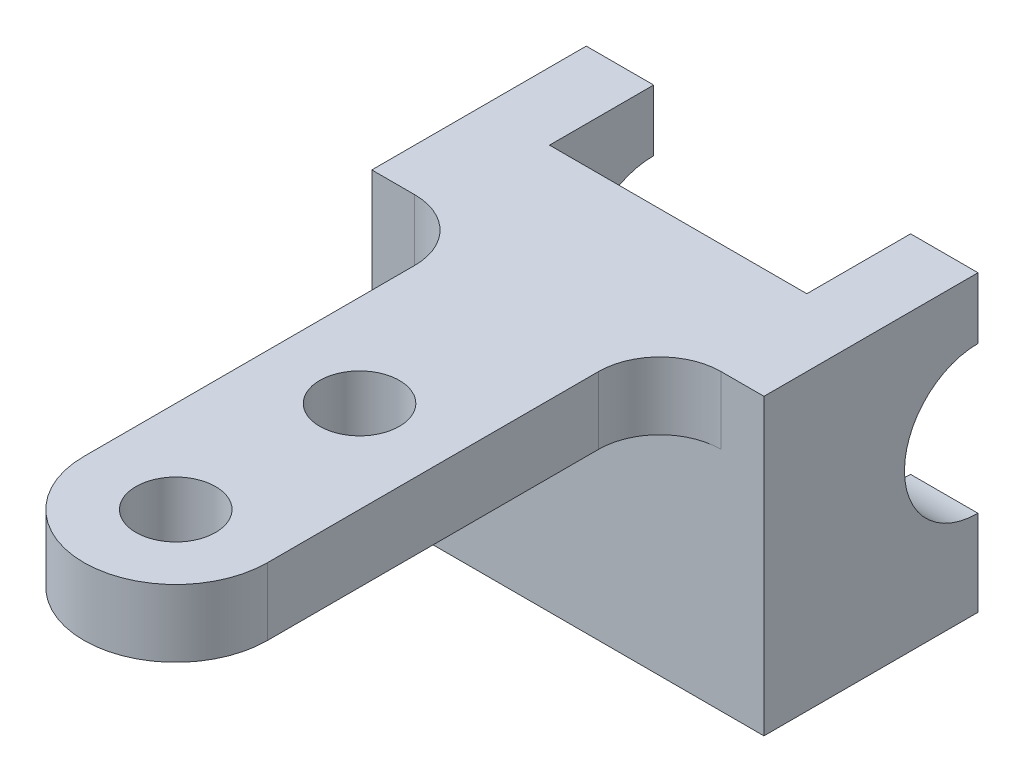
ISO-10303-21;
HEADER;
FILE_DESCRIPTION(('STEP AP214'),'2;1');
FILE_NAME('part.step','',(''),(''),'','','');
FILE_SCHEMA(('AUTOMOTIVE_DESIGN { 1 0 10303 214 1 1 1 1 }'));
ENDSEC;
DATA;
#1=APPLICATION_CONTEXT('core data for automotive mechanical design processes');
#2=APPLICATION_PROTOCOL_DEFINITION('international standard','automotive_design',2000,#1);
#3=PRODUCT_CONTEXT('',#1,'mechanical');
#4=PRODUCT('Part','Part','',(#3));
#5=PRODUCT_RELATED_PRODUCT_CATEGORY('part','',(#4));
#6=PRODUCT_DEFINITION_FORMATION('','',#4);
#7=PRODUCT_DEFINITION_CONTEXT('part definition',#1,'design');
#8=PRODUCT_DEFINITION('design','',#6,#7);
#9=PRODUCT_DEFINITION_SHAPE('','',#8);
#10=(LENGTH_UNIT() NAMED_UNIT(*) SI_UNIT(.MILLI.,.METRE.));
#11=(NAMED_UNIT(*) PLANE_ANGLE_UNIT() SI_UNIT($,.RADIAN.));
#12=(NAMED_UNIT(*) SI_UNIT($,.STERADIAN.) SOLID_ANGLE_UNIT());
#13=UNCERTAINTY_MEASURE_WITH_UNIT(LENGTH_MEASURE(1.E-05),#10,'distance_accuracy_value','');
#14=(GEOMETRIC_REPRESENTATION_CONTEXT(3) GLOBAL_UNCERTAINTY_ASSIGNED_CONTEXT((#13)) GLOBAL_UNIT_ASSIGNED_CONTEXT((#10,
#11,#12)) REPRESENTATION_CONTEXT('',''));
#15=CARTESIAN_POINT('',(0.,0.,0.));
#16=DIRECTION('',(0.,0.,1.));
#17=DIRECTION('',(1.,0.,0.));
#18=AXIS2_PLACEMENT_3D('',#15,#16,#17);
#19=CARTESIAN_POINT('',(32.,11.,-64.));
#20=DIRECTION('',(-1.,0.,0.));
#21=DIRECTION('',(0.,0.,1.));
#22=AXIS2_PLACEMENT_3D('',#19,#20,#21);
#23=PLANE('',#22);
#24=CARTESIAN_POINT('',(32.000012,-11.,-98.9340644485926));
#25=DIRECTION('',(1.,0.,0.));
#26=DIRECTION('',(0.,1.,2.23257407931203E-09));
#27=AXIS2_PLACEMENT_3D('',#24,#25,#26);
#28=CIRCLE('',#27,12.);
#29=CARTESIAN_POINT('',(32.000006,0.99999999999999,-98.9340644351971));
#30=VERTEX_POINT('',#29);
#31=CARTESIAN_POINT('',(32.000006,-23.,-98.9340644560229));
#32=VERTEX_POINT('',#31);
#33=EDGE_CURVE('E184',#30,#32,#28,.T.);
#34=ORIENTED_EDGE('',*,*,#33,.F.);
#35=DIRECTION('',(0.,-1.,0.));
#36=VECTOR('',#35,1.);
#37=CARTESIAN_POINT('',(32.,11.,-98.9340644485926));
#38=LINE('',#37,#36);
#39=CARTESIAN_POINT('',(32.,11.,-98.9340644485926));
#40=VERTEX_POINT('',#39);
#41=EDGE_CURVE('E216',#40,#30,#38,.T.);
#42=ORIENTED_EDGE('',*,*,#41,.F.);
#43=DIRECTION('',(0.,0.,-1.));
#44=VECTOR('',#43,1.);
#45=CARTESIAN_POINT('',(32.,11.,-64.));
#46=LINE('',#45,#44);
#47=CARTESIAN_POINT('',(32.,11.,-64.));
#48=VERTEX_POINT('',#47);
#49=EDGE_CURVE('E253',#48,#40,#46,.T.);
#50=ORIENTED_EDGE('',*,*,#49,.F.);
#51=DIRECTION('',(0.,-1.,0.));
#52=VECTOR('',#51,1.);
#53=CARTESIAN_POINT('',(32.,11.,-64.));
#54=LINE('',#53,#52);
#55=CARTESIAN_POINT('',(32.,-37.,-64.));
#56=VERTEX_POINT('',#55);
#57=EDGE_CURVE('E211',#48,#56,#54,.T.);
#58=ORIENTED_EDGE('',*,*,#57,.T.);
#59=DIRECTION('',(0.,0.,1.));
#60=VECTOR('',#59,1.);
#61=CARTESIAN_POINT('',(32.,-37.,-64.));
#62=LINE('',#61,#60);
#63=CARTESIAN_POINT('',(32.,-37.,-98.9340644485926));
#64=VERTEX_POINT('',#63);
#65=EDGE_CURVE('E246',#64,#56,#62,.T.);
#66=ORIENTED_EDGE('',*,*,#65,.F.);
#67=EDGE_CURVE('E208',#32,#64,#38,.T.);
#68=ORIENTED_EDGE('',*,*,#67,.F.);
#69=EDGE_LOOP('',(#34,#42,#50,#58,#66,#68));
#70=FACE_BOUND('',#69,.T.);
#71=ADVANCED_FACE('F39',(#70),#23,.F.);
#72=CARTESIAN_POINT('',(32.,11.,-98.9340644485926));
#73=DIRECTION('',(0.,0.,1.));
#74=DIRECTION('',(1.,0.,0.));
#75=AXIS2_PLACEMENT_3D('',#72,#73,#74);
#76=PLANE('',#75);
#77=DIRECTION('',(0.,-1.,0.));
#78=VECTOR('',#77,1.);
#79=CARTESIAN_POINT('',(21.,11.,-98.9340644485926));
#80=LINE('',#79,#78);
#81=CARTESIAN_POINT('',(21.,-23.,-98.9340644485926));
#82=VERTEX_POINT('',#81);
#83=CARTESIAN_POINT('',(21.,-37.,-98.9340644485926));
#84=VERTEX_POINT('',#83);
#85=EDGE_CURVE('E204',#82,#84,#80,.T.);
#86=ORIENTED_EDGE('',*,*,#85,.F.);
#87=DIRECTION('',(1.,0.,0.));
#88=VECTOR('',#87,1.);
#89=CARTESIAN_POINT('',(-32.,-23.,-98.9340644485926));
#90=LINE('',#89,#88);
#91=EDGE_CURVE('E59',#82,#32,#90,.T.);
#92=ORIENTED_EDGE('',*,*,#91,.T.);
#93=ORIENTED_EDGE('',*,*,#67,.T.);
#94=DIRECTION('',(1.,0.,0.));
#95=VECTOR('',#94,1.);
#96=CARTESIAN_POINT('',(32.,-37.,-98.9340644485926));
#97=LINE('',#96,#95);
#98=EDGE_CURVE('E265',#84,#64,#97,.T.);
#99=ORIENTED_EDGE('',*,*,#98,.F.);
#100=EDGE_LOOP('',(#86,#92,#93,#99));
#101=FACE_BOUND('',#100,.T.);
#102=ADVANCED_FACE('F351',(#101),#76,.F.);
#103=CARTESIAN_POINT('',(-21.,11.,-99.));
#104=DIRECTION('',(0.,0.,1.));
#105=DIRECTION('',(1.,0.,0.));
#106=AXIS2_PLACEMENT_3D('',#103,#104,#105);
#107=PLANE('',#106);
#108=DIRECTION('',(0.,-1.,0.));
#109=VECTOR('',#108,1.);
#110=CARTESIAN_POINT('',(-32.,11.,-99.));
#111=LINE('',#110,#109);
#112=CARTESIAN_POINT('',(-32.,-22.9998188529269,-99.));
#113=VERTEX_POINT('',#112);
#114=CARTESIAN_POINT('',(-32.,-37.,-99.));
#115=VERTEX_POINT('',#114);
#116=EDGE_CURVE('E179',#113,#115,#111,.T.);
#117=ORIENTED_EDGE('',*,*,#116,.F.);
#118=DIRECTION('',(1.,0.,0.));
#119=VECTOR('',#118,1.);
#120=CARTESIAN_POINT('',(-32.,-22.9998188529269,-99.));
#121=LINE('',#120,#119);
#122=CARTESIAN_POINT('',(-21.,-22.9998188529269,-99.));
#123=VERTEX_POINT('',#122);
#124=EDGE_CURVE('E164',#113,#123,#121,.T.);
#125=ORIENTED_EDGE('',*,*,#124,.T.);
#126=DIRECTION('',(0.,-1.,0.));
#127=VECTOR('',#126,1.);
#128=CARTESIAN_POINT('',(-21.,11.,-99.));
#129=LINE('',#128,#127);
#130=CARTESIAN_POINT('',(-21.,-37.,-99.));
#131=VERTEX_POINT('',#130);
#132=EDGE_CURVE('E195',#123,#131,#129,.T.);
#133=ORIENTED_EDGE('',*,*,#132,.T.);
#134=DIRECTION('',(1.,0.,0.));
#135=VECTOR('',#134,1.);
#136=CARTESIAN_POINT('',(-21.,-37.,-99.));
#137=LINE('',#136,#135);
#138=EDGE_CURVE('E186',#115,#131,#137,.T.);
#139=ORIENTED_EDGE('',*,*,#138,.F.);
#140=EDGE_LOOP('',(#117,#125,#133,#139));
#141=FACE_BOUND('',#140,.T.);
#142=ADVANCED_FACE('F188',(#141),#107,.F.);
#143=CARTESIAN_POINT('',(0.,0.,0.));
#144=DIRECTION('',(0.,1.,0.));
#145=DIRECTION('',(0.,0.,1.));
#146=AXIS2_PLACEMENT_3D('',#143,#144,#145);
#147=PLANE('',#146);
#148=CARTESIAN_POINT('',(0.,0.,-30.));
#149=DIRECTION('',(0.,1.,0.));
#150=DIRECTION('',(0.,0.,1.));
#151=AXIS2_PLACEMENT_3D('',#148,#149,#150);
#152=CIRCLE('',#151,6.5);
#153=CARTESIAN_POINT('',(0.,0.,-23.5));
#154=VERTEX_POINT('',#153);
#155=EDGE_CURVE('E270',#154,#154,#152,.T.);
#156=ORIENTED_EDGE('',*,*,#155,.T.);
#157=EDGE_LOOP('',(#156));
#158=FACE_BOUND('',#157,.T.);
#159=CARTESIAN_POINT('',(0.,0.,0.));
#160=DIRECTION('',(0.,1.,0.));
#161=DIRECTION('',(0.,0.,1.));
#162=AXIS2_PLACEMENT_3D('',#159,#160,#161);
#163=CIRCLE('',#162,6.5);
#164=CARTESIAN_POINT('',(0.,0.,6.5));
#165=VERTEX_POINT('',#164);
#166=EDGE_CURVE('E274',#165,#165,#163,.T.);
#167=ORIENTED_EDGE('',*,*,#166,.T.);
#168=EDGE_LOOP('',(#167));
#169=FACE_BOUND('',#168,.T.);
#170=DIRECTION('',(-1.,0.,0.));
#171=VECTOR('',#170,1.);
#172=CARTESIAN_POINT('',(-32.,0.,-64.));
#173=LINE('',#172,#171);
#174=CARTESIAN_POINT('',(25.,0.,-64.));
#175=VERTEX_POINT('',#174);
#176=CARTESIAN_POINT('',(-25.,0.,-64.));
#177=VERTEX_POINT('',#176);
#178=EDGE_CURVE('E231',#175,#177,#173,.T.);
#179=ORIENTED_EDGE('',*,*,#178,.F.);
#180=CARTESIAN_POINT('',(25.,0.,-54.));
#181=DIRECTION('',(0.,1.,0.));
#182=DIRECTION('',(0.,0.,1.));
#183=AXIS2_PLACEMENT_3D('',#180,#181,#182);
#184=CIRCLE('',#183,10.);
#185=CARTESIAN_POINT('',(15.,0.,-54.));
#186=VERTEX_POINT('',#185);
#187=EDGE_CURVE('E49',#175,#186,#184,.T.);
#188=ORIENTED_EDGE('',*,*,#187,.T.);
#189=DIRECTION('',(0.,0.,-1.));
#190=VECTOR('',#189,1.);
#191=CARTESIAN_POINT('',(15.,0.,0.));
#192=LINE('',#191,#190);
#193=CARTESIAN_POINT('',(15.,0.,0.));
#194=VERTEX_POINT('',#193);
#195=EDGE_CURVE('E313',#194,#186,#192,.T.);
#196=ORIENTED_EDGE('',*,*,#195,.F.);
#197=CARTESIAN_POINT('',(0.,0.,0.));
#198=DIRECTION('',(0.,1.,0.));
#199=DIRECTION('',(0.,0.,1.));
#200=AXIS2_PLACEMENT_3D('',#197,#198,#199);
#201=CIRCLE('',#200,15.);
#202=CARTESIAN_POINT('',(-15.,0.,0.));
#203=VERTEX_POINT('',#202);
#204=EDGE_CURVE('E278',#203,#194,#201,.T.);
#205=ORIENTED_EDGE('',*,*,#204,.F.);
#206=DIRECTION('',(0.,0.,1.));
#207=VECTOR('',#206,1.);
#208=CARTESIAN_POINT('',(-15.,0.,0.));
#209=LINE('',#208,#207);
#210=CARTESIAN_POINT('',(-15.,0.,-54.));
#211=VERTEX_POINT('',#210);
#212=EDGE_CURVE('E290',#211,#203,#209,.T.);
#213=ORIENTED_EDGE('',*,*,#212,.F.);
#214=CARTESIAN_POINT('',(-25.,0.,-54.));
#215=DIRECTION('',(0.,1.,0.));
#216=DIRECTION('',(0.,0.,1.));
#217=AXIS2_PLACEMENT_3D('',#214,#215,#216);
#218=CIRCLE('',#217,10.);
#219=EDGE_CURVE('E225',#211,#177,#218,.T.);
#220=ORIENTED_EDGE('',*,*,#219,.T.);
#221=EDGE_LOOP('',(#179,#188,#196,#205,#213,#220));
#222=FACE_BOUND('',#221,.T.);
#223=ADVANCED_FACE('F323',(#158,#169,#222),#147,.F.);
#224=CARTESIAN_POINT('',(0.,11.,0.));
#225=DIRECTION('',(0.,1.,0.));
#226=DIRECTION('',(0.,0.,1.));
#227=AXIS2_PLACEMENT_3D('',#224,#225,#226);
#228=PLANE('',#227);
#229=CARTESIAN_POINT('',(0.,11.,0.));
#230=DIRECTION('',(0.,1.,0.));
#231=DIRECTION('',(0.,0.,1.));
#232=AXIS2_PLACEMENT_3D('',#229,#230,#231);
#233=CIRCLE('',#232,6.5);
#234=CARTESIAN_POINT('',(0.,11.,6.5));
#235=VERTEX_POINT('',#234);
#236=EDGE_CURVE('E280',#235,#235,#233,.T.);
#237=ORIENTED_EDGE('',*,*,#236,.F.);
#238=EDGE_LOOP('',(#237));
#239=FACE_BOUND('',#238,.T.);
#240=CARTESIAN_POINT('',(0.,11.,0.));
#241=DIRECTION('',(0.,1.,0.));
#242=DIRECTION('',(0.,0.,1.));
#243=AXIS2_PLACEMENT_3D('',#240,#241,#242);
#244=CIRCLE('',#243,15.);
#245=CARTESIAN_POINT('',(-15.,11.,0.));
#246=VERTEX_POINT('',#245);
#247=CARTESIAN_POINT('',(15.,11.,0.));
#248=VERTEX_POINT('',#247);
#249=EDGE_CURVE('E281',#246,#248,#244,.T.);
#250=ORIENTED_EDGE('',*,*,#249,.T.);
#251=DIRECTION('',(0.,0.,-1.));
#252=VECTOR('',#251,1.);
#253=CARTESIAN_POINT('',(15.,11.,0.));
#254=LINE('',#253,#252);
#255=CARTESIAN_POINT('',(15.,11.,-54.));
#256=VERTEX_POINT('',#255);
#257=EDGE_CURVE('E287',#248,#256,#254,.T.);
#258=ORIENTED_EDGE('',*,*,#257,.T.);
#259=CARTESIAN_POINT('',(25.,11.,-54.));
#260=DIRECTION('',(0.,1.,0.));
#261=DIRECTION('',(0.,0.,1.));
#262=AXIS2_PLACEMENT_3D('',#259,#260,#261);
#263=CIRCLE('',#262,10.);
#264=CARTESIAN_POINT('',(25.,11.,-64.));
#265=VERTEX_POINT('',#264);
#266=EDGE_CURVE('E11',#256,#265,#263,.F.);
#267=ORIENTED_EDGE('',*,*,#266,.T.);
#268=DIRECTION('',(1.,0.,0.));
#269=VECTOR('',#268,1.);
#270=CARTESIAN_POINT('',(15.,11.,-64.));
#271=LINE('',#270,#269);
#272=EDGE_CURVE('E288',#265,#48,#271,.T.);
#273=ORIENTED_EDGE('',*,*,#272,.T.);
#274=ORIENTED_EDGE('',*,*,#49,.T.);
#275=DIRECTION('',(-1.,0.,0.));
#276=VECTOR('',#275,1.);
#277=CARTESIAN_POINT('',(32.,11.,-98.9340644485926));
#278=LINE('',#277,#276);
#279=CARTESIAN_POINT('',(21.,11.,-98.9340644485926));
#280=VERTEX_POINT('',#279);
#281=EDGE_CURVE('E291',#40,#280,#278,.T.);
#282=ORIENTED_EDGE('',*,*,#281,.T.);
#283=DIRECTION('',(0.,0.,1.));
#284=VECTOR('',#283,1.);
#285=CARTESIAN_POINT('',(21.,11.,-98.9340644485926));
#286=LINE('',#285,#284);
#287=CARTESIAN_POINT('',(21.,11.,-82.));
#288=VERTEX_POINT('',#287);
#289=EDGE_CURVE('E293',#280,#288,#286,.T.);
#290=ORIENTED_EDGE('',*,*,#289,.T.);
#291=DIRECTION('',(-1.,0.,0.));
#292=VECTOR('',#291,1.);
#293=CARTESIAN_POINT('',(21.,11.,-82.));
#294=LINE('',#293,#292);
#295=CARTESIAN_POINT('',(-21.,11.,-82.));
#296=VERTEX_POINT('',#295);
#297=EDGE_CURVE('E300',#288,#296,#294,.T.);
#298=ORIENTED_EDGE('',*,*,#297,.T.);
#299=DIRECTION('',(0.,0.,-1.));
#300=VECTOR('',#299,1.);
#301=CARTESIAN_POINT('',(-21.,11.,-82.));
#302=LINE('',#301,#300);
#303=CARTESIAN_POINT('',(-21.,11.,-99.));
#304=VERTEX_POINT('',#303);
#305=EDGE_CURVE('E299',#296,#304,#302,.T.);
#306=ORIENTED_EDGE('',*,*,#305,.T.);
#307=DIRECTION('',(-1.,0.,0.));
#308=VECTOR('',#307,1.);
#309=CARTESIAN_POINT('',(-21.,11.,-99.));
#310=LINE('',#309,#308);
#311=CARTESIAN_POINT('',(-32.,11.,-99.));
#312=VERTEX_POINT('',#311);
#313=EDGE_CURVE('E302',#304,#312,#310,.T.);
#314=ORIENTED_EDGE('',*,*,#313,.T.);
#315=DIRECTION('',(0.,0.,1.));
#316=VECTOR('',#315,1.);
#317=CARTESIAN_POINT('',(-32.,11.,-99.));
#318=LINE('',#317,#316);
#319=CARTESIAN_POINT('',(-32.,11.,-64.));
#320=VERTEX_POINT('',#319);
#321=EDGE_CURVE('E304',#312,#320,#318,.T.);
#322=ORIENTED_EDGE('',*,*,#321,.T.);
#323=DIRECTION('',(1.,0.,0.));
#324=VECTOR('',#323,1.);
#325=CARTESIAN_POINT('',(-32.,11.,-64.));
#326=LINE('',#325,#324);
#327=CARTESIAN_POINT('',(-25.,11.,-64.));
#328=VERTEX_POINT('',#327);
#329=EDGE_CURVE('E303',#320,#328,#326,.T.);
#330=ORIENTED_EDGE('',*,*,#329,.T.);
#331=CARTESIAN_POINT('',(-25.,11.,-54.));
#332=DIRECTION('',(0.,1.,0.));
#333=DIRECTION('',(0.,0.,1.));
#334=AXIS2_PLACEMENT_3D('',#331,#332,#333);
#335=CIRCLE('',#334,10.);
#336=CARTESIAN_POINT('',(-15.,11.,-54.));
#337=VERTEX_POINT('',#336);
#338=EDGE_CURVE('E219',#328,#337,#335,.F.);
#339=ORIENTED_EDGE('',*,*,#338,.T.);
#340=DIRECTION('',(0.,0.,1.));
#341=VECTOR('',#340,1.);
#342=CARTESIAN_POINT('',(-15.,11.,0.));
#343=LINE('',#342,#341);
#344=EDGE_CURVE('E306',#337,#246,#343,.T.);
#345=ORIENTED_EDGE('',*,*,#344,.T.);
#346=EDGE_LOOP('',(#250,#258,#267,#273,#274,#282,#290,#298,#306,#314,#322,#330,#339,#345));
#347=FACE_BOUND('',#346,.T.);
#348=CARTESIAN_POINT('',(0.,11.,-30.));
#349=DIRECTION('',(0.,1.,0.));
#350=DIRECTION('',(0.,0.,1.));
#351=AXIS2_PLACEMENT_3D('',#348,#349,#350);
#352=CIRCLE('',#351,6.5);
#353=CARTESIAN_POINT('',(0.,11.,-23.5));
#354=VERTEX_POINT('',#353);
#355=EDGE_CURVE('E269',#354,#354,#352,.T.);
#356=ORIENTED_EDGE('',*,*,#355,.F.);
#357=EDGE_LOOP('',(#356));
#358=FACE_BOUND('',#357,.T.);
#359=ADVANCED_FACE('F332',(#239,#347,#358),#228,.T.);
#360=CARTESIAN_POINT('',(0.,11.,0.));
#361=DIRECTION('',(0.,-1.,0.));
#362=DIRECTION('',(0.,0.,-1.));
#363=AXIS2_PLACEMENT_3D('',#360,#361,#362);
#364=CYLINDRICAL_SURFACE('',#363,15.);
#365=ORIENTED_EDGE('',*,*,#204,.T.);
#366=DIRECTION('',(0.,-1.,0.));
#367=VECTOR('',#366,1.);
#368=CARTESIAN_POINT('',(15.,11.,0.));
#369=LINE('',#368,#367);
#370=EDGE_CURVE('E233',#248,#194,#369,.T.);
#371=ORIENTED_EDGE('',*,*,#370,.F.);
#372=ORIENTED_EDGE('',*,*,#249,.F.);
#373=DIRECTION('',(0.,-1.,0.));
#374=VECTOR('',#373,1.);
#375=CARTESIAN_POINT('',(-15.,11.,0.));
#376=LINE('',#375,#374);
#377=EDGE_CURVE('E194',#246,#203,#376,.T.);
#378=ORIENTED_EDGE('',*,*,#377,.T.);
#379=EDGE_LOOP('',(#365,#371,#372,#378));
#380=FACE_BOUND('',#379,.T.);
#381=ADVANCED_FACE('F318',(#380),#364,.T.);
#382=CARTESIAN_POINT('',(15.,11.,0.));
#383=DIRECTION('',(-1.,0.,0.));
#384=DIRECTION('',(0.,0.,1.));
#385=AXIS2_PLACEMENT_3D('',#382,#383,#384);
#386=PLANE('',#385);
#387=ORIENTED_EDGE('',*,*,#195,.T.);
#388=DIRECTION('',(0.,-1.,0.));
#389=VECTOR('',#388,1.);
#390=CARTESIAN_POINT('',(15.,11.,-54.));
#391=LINE('',#390,#389);
#392=EDGE_CURVE('E223',#186,#256,#391,.F.);
#393=ORIENTED_EDGE('',*,*,#392,.T.);
#394=ORIENTED_EDGE('',*,*,#257,.F.);
#395=ORIENTED_EDGE('',*,*,#370,.T.);
#396=EDGE_LOOP('',(#387,#393,#394,#395));
#397=FACE_BOUND('',#396,.T.);
#398=ADVANCED_FACE('F326',(#397),#386,.F.);
#399=ORIENTED_EDGE('',*,*,#41,.T.);
#400=DIRECTION('',(1.,0.,0.));
#401=VECTOR('',#400,1.);
#402=CARTESIAN_POINT('',(-32.,0.99999999999999,-98.9340644485926));
#403=LINE('',#402,#401);
#404=CARTESIAN_POINT('',(21.,0.99999999999999,-98.9340644485926));
#405=VERTEX_POINT('',#404);
#406=EDGE_CURVE('E417',#30,#405,#403,.F.);
#407=ORIENTED_EDGE('',*,*,#406,.T.);
#408=EDGE_CURVE('E202',#280,#405,#80,.T.);
#409=ORIENTED_EDGE('',*,*,#408,.F.);
#410=ORIENTED_EDGE('',*,*,#281,.F.);
#411=EDGE_LOOP('',(#399,#407,#409,#410));
#412=FACE_BOUND('',#411,.T.);
#413=ADVANCED_FACE('F358',(#412),#76,.F.);
#414=CARTESIAN_POINT('',(21.,11.,-98.9340644485926));
#415=DIRECTION('',(1.,0.,0.));
#416=DIRECTION('',(0.,0.,-1.));
#417=AXIS2_PLACEMENT_3D('',#414,#415,#416);
#418=PLANE('',#417);
#419=ORIENTED_EDGE('',*,*,#408,.T.);
#420=CARTESIAN_POINT('',(21.,-11.,-98.9340644485926));
#421=DIRECTION('',(1.,0.,0.));
#422=DIRECTION('',(0.,0.,-1.));
#423=AXIS2_PLACEMENT_3D('',#420,#421,#422);
#424=CIRCLE('',#423,12.);
#425=EDGE_CURVE('E175',#405,#82,#424,.T.);
#426=ORIENTED_EDGE('',*,*,#425,.T.);
#427=ORIENTED_EDGE('',*,*,#85,.T.);
#428=DIRECTION('',(0.,0.,-1.));
#429=VECTOR('',#428,1.);
#430=CARTESIAN_POINT('',(21.,-37.,-98.9340644485926));
#431=LINE('',#430,#429);
#432=CARTESIAN_POINT('',(21.,-37.,-82.));
#433=VERTEX_POINT('',#432);
#434=EDGE_CURVE('E444',#433,#84,#431,.T.);
#435=ORIENTED_EDGE('',*,*,#434,.F.);
#436=DIRECTION('',(0.,-1.,0.));
#437=VECTOR('',#436,1.);
#438=CARTESIAN_POINT('',(21.,11.,-82.));
#439=LINE('',#438,#437);
#440=EDGE_CURVE('E205',#288,#433,#439,.T.);
#441=ORIENTED_EDGE('',*,*,#440,.F.);
#442=ORIENTED_EDGE('',*,*,#289,.F.);
#443=EDGE_LOOP('',(#419,#426,#427,#435,#441,#442));
#444=FACE_BOUND('',#443,.T.);
#445=ADVANCED_FACE('F453',(#444),#418,.F.);
#446=CARTESIAN_POINT('',(21.,11.,-82.));
#447=DIRECTION('',(0.,0.,1.));
#448=DIRECTION('',(1.,0.,0.));
#449=AXIS2_PLACEMENT_3D('',#446,#447,#448);
#450=PLANE('',#449);
#451=ORIENTED_EDGE('',*,*,#440,.T.);
#452=DIRECTION('',(1.,0.,0.));
#453=VECTOR('',#452,1.);
#454=CARTESIAN_POINT('',(21.,-37.,-82.));
#455=LINE('',#454,#453);
#456=CARTESIAN_POINT('',(-21.,-37.,-82.));
#457=VERTEX_POINT('',#456);
#458=EDGE_CURVE('E439',#457,#433,#455,.T.);
#459=ORIENTED_EDGE('',*,*,#458,.F.);
#460=DIRECTION('',(0.,-1.,0.));
#461=VECTOR('',#460,1.);
#462=CARTESIAN_POINT('',(-21.,11.,-82.));
#463=LINE('',#462,#461);
#464=EDGE_CURVE('E199',#296,#457,#463,.T.);
#465=ORIENTED_EDGE('',*,*,#464,.F.);
#466=ORIENTED_EDGE('',*,*,#297,.F.);
#467=EDGE_LOOP('',(#451,#459,#465,#466));
#468=FACE_BOUND('',#467,.T.);
#469=ADVANCED_FACE('F410',(#468),#450,.F.);
#470=CARTESIAN_POINT('',(-21.,11.,-82.));
#471=DIRECTION('',(-1.,0.,0.));
#472=DIRECTION('',(0.,0.,1.));
#473=AXIS2_PLACEMENT_3D('',#470,#471,#472);
#474=PLANE('',#473);
#475=ORIENTED_EDGE('',*,*,#132,.F.);
#476=CARTESIAN_POINT('',(-21.,-11.,-98.9340644485926));
#477=DIRECTION('',(-1.,0.,0.));
#478=DIRECTION('',(0.,0.,1.));
#479=AXIS2_PLACEMENT_3D('',#476,#477,#478);
#480=CIRCLE('',#479,12.);
#481=CARTESIAN_POINT('',(-21.,0.999818852926921,-99.));
#482=VERTEX_POINT('',#481);
#483=EDGE_CURVE('E169',#123,#482,#480,.T.);
#484=ORIENTED_EDGE('',*,*,#483,.T.);
#485=EDGE_CURVE('E197',#304,#482,#129,.T.);
#486=ORIENTED_EDGE('',*,*,#485,.F.);
#487=ORIENTED_EDGE('',*,*,#305,.F.);
#488=ORIENTED_EDGE('',*,*,#464,.T.);
#489=DIRECTION('',(0.,0.,1.));
#490=VECTOR('',#489,1.);
#491=CARTESIAN_POINT('',(-21.,-37.,-82.));
#492=LINE('',#491,#490);
#493=EDGE_CURVE('E440',#131,#457,#492,.T.);
#494=ORIENTED_EDGE('',*,*,#493,.F.);
#495=EDGE_LOOP('',(#475,#484,#486,#487,#488,#494));
#496=FACE_BOUND('',#495,.T.);
#497=ADVANCED_FACE('F402',(#496),#474,.F.);
#498=ORIENTED_EDGE('',*,*,#485,.T.);
#499=DIRECTION('',(1.,0.,0.));
#500=VECTOR('',#499,1.);
#501=CARTESIAN_POINT('',(-32.,0.999818852926921,-99.));
#502=LINE('',#501,#500);
#503=CARTESIAN_POINT('',(-32.,0.999818852926921,-99.));
#504=VERTEX_POINT('',#503);
#505=EDGE_CURVE('E181',#482,#504,#502,.F.);
#506=ORIENTED_EDGE('',*,*,#505,.T.);
#507=EDGE_CURVE('E185',#312,#504,#111,.T.);
#508=ORIENTED_EDGE('',*,*,#507,.F.);
#509=ORIENTED_EDGE('',*,*,#313,.F.);
#510=EDGE_LOOP('',(#498,#506,#508,#509));
#511=FACE_BOUND('',#510,.T.);
#512=ADVANCED_FACE('F386',(#511),#107,.F.);
#513=CARTESIAN_POINT('',(-32.,11.,-99.));
#514=DIRECTION('',(1.,0.,0.));
#515=DIRECTION('',(0.,0.,-1.));
#516=AXIS2_PLACEMENT_3D('',#513,#514,#515);
#517=PLANE('',#516);
#518=ORIENTED_EDGE('',*,*,#507,.T.);
#519=CARTESIAN_POINT('',(-32.,-11.,-98.9340644485926));
#520=DIRECTION('',(1.,0.,0.));
#521=DIRECTION('',(0.,0.,-1.));
#522=AXIS2_PLACEMENT_3D('',#519,#520,#521);
#523=CIRCLE('',#522,12.);
#524=EDGE_CURVE('E67',#504,#113,#523,.T.);
#525=ORIENTED_EDGE('',*,*,#524,.T.);
#526=ORIENTED_EDGE('',*,*,#116,.T.);
#527=DIRECTION('',(0.,0.,-1.));
#528=VECTOR('',#527,1.);
#529=CARTESIAN_POINT('',(-32.,-37.,-99.));
#530=LINE('',#529,#528);
#531=CARTESIAN_POINT('',(-32.,-37.,-64.));
#532=VERTEX_POINT('',#531);
#533=EDGE_CURVE('E421',#532,#115,#530,.T.);
#534=ORIENTED_EDGE('',*,*,#533,.F.);
#535=DIRECTION('',(0.,-1.,0.));
#536=VECTOR('',#535,1.);
#537=CARTESIAN_POINT('',(-32.,11.,-64.));
#538=LINE('',#537,#536);
#539=EDGE_CURVE('E187',#320,#532,#538,.T.);
#540=ORIENTED_EDGE('',*,*,#539,.F.);
#541=ORIENTED_EDGE('',*,*,#321,.F.);
#542=EDGE_LOOP('',(#518,#525,#526,#534,#540,#541));
#543=FACE_BOUND('',#542,.T.);
#544=ADVANCED_FACE('F177',(#543),#517,.F.);
#545=CARTESIAN_POINT('',(-32.,11.,-64.));
#546=DIRECTION('',(0.,0.,-1.));
#547=DIRECTION('',(-1.,0.,0.));
#548=AXIS2_PLACEMENT_3D('',#545,#546,#547);
#549=PLANE('',#548);
#550=ORIENTED_EDGE('',*,*,#178,.T.);
#551=DIRECTION('',(0.,-1.,0.));
#552=VECTOR('',#551,1.);
#553=CARTESIAN_POINT('',(-25.,11.,-64.));
#554=LINE('',#553,#552);
#555=EDGE_CURVE('E230',#177,#328,#554,.F.);
#556=ORIENTED_EDGE('',*,*,#555,.T.);
#557=ORIENTED_EDGE('',*,*,#329,.F.);
#558=ORIENTED_EDGE('',*,*,#539,.T.);
#559=DIRECTION('',(-1.,0.,0.));
#560=VECTOR('',#559,1.);
#561=CARTESIAN_POINT('',(-32.,-37.,-64.));
#562=LINE('',#561,#560);
#563=EDGE_CURVE('E259',#56,#532,#562,.T.);
#564=ORIENTED_EDGE('',*,*,#563,.F.);
#565=ORIENTED_EDGE('',*,*,#57,.F.);
#566=ORIENTED_EDGE('',*,*,#272,.F.);
#567=DIRECTION('',(0.,-1.,0.));
#568=VECTOR('',#567,1.);
#569=CARTESIAN_POINT('',(25.,0.,-64.));
#570=LINE('',#569,#568);
#571=EDGE_CURVE('E229',#265,#175,#570,.T.);
#572=ORIENTED_EDGE('',*,*,#571,.T.);
#573=EDGE_LOOP('',(#550,#556,#557,#558,#564,#565,#566,#572));
#574=FACE_BOUND('',#573,.T.);
#575=ADVANCED_FACE('F262',(#574),#549,.F.);
#576=CARTESIAN_POINT('',(-15.,11.,0.));
#577=DIRECTION('',(1.,0.,0.));
#578=DIRECTION('',(0.,0.,-1.));
#579=AXIS2_PLACEMENT_3D('',#576,#577,#578);
#580=PLANE('',#579);
#581=ORIENTED_EDGE('',*,*,#344,.F.);
#582=DIRECTION('',(0.,-1.,0.));
#583=VECTOR('',#582,1.);
#584=CARTESIAN_POINT('',(-15.,0.,-54.));
#585=LINE('',#584,#583);
#586=EDGE_CURVE('E235',#337,#211,#585,.T.);
#587=ORIENTED_EDGE('',*,*,#586,.T.);
#588=ORIENTED_EDGE('',*,*,#212,.T.);
#589=ORIENTED_EDGE('',*,*,#377,.F.);
#590=EDGE_LOOP('',(#581,#587,#588,#589));
#591=FACE_BOUND('',#590,.T.);
#592=ADVANCED_FACE('F336',(#591),#580,.F.);
#593=CARTESIAN_POINT('',(0.,11.,0.));
#594=DIRECTION('',(0.,-1.,0.));
#595=DIRECTION('',(0.,0.,-1.));
#596=AXIS2_PLACEMENT_3D('',#593,#594,#595);
#597=CYLINDRICAL_SURFACE('',#596,6.5);
#598=ORIENTED_EDGE('',*,*,#236,.T.);
#599=EDGE_LOOP('',(#598));
#600=FACE_BOUND('',#599,.T.);
#601=ORIENTED_EDGE('',*,*,#166,.F.);
#602=EDGE_LOOP('',(#601));
#603=FACE_BOUND('',#602,.T.);
#604=ADVANCED_FACE('F337',(#600,#603),#597,.F.);
#605=CARTESIAN_POINT('',(0.,11.,-30.));
#606=DIRECTION('',(0.,-1.,0.));
#607=DIRECTION('',(0.,0.,-1.));
#608=AXIS2_PLACEMENT_3D('',#605,#606,#607);
#609=CYLINDRICAL_SURFACE('',#608,6.5);
#610=ORIENTED_EDGE('',*,*,#355,.T.);
#611=EDGE_LOOP('',(#610));
#612=FACE_BOUND('',#611,.T.);
#613=ORIENTED_EDGE('',*,*,#155,.F.);
#614=EDGE_LOOP('',(#613));
#615=FACE_BOUND('',#614,.T.);
#616=ADVANCED_FACE('F350',(#612,#615),#609,.F.);
#617=CARTESIAN_POINT('',(0.,-37.,0.));
#618=DIRECTION('',(0.,1.,0.));
#619=DIRECTION('',(0.,0.,1.));
#620=AXIS2_PLACEMENT_3D('',#617,#618,#619);
#621=PLANE('',#620);
#622=ORIENTED_EDGE('',*,*,#533,.T.);
#623=ORIENTED_EDGE('',*,*,#138,.T.);
#624=ORIENTED_EDGE('',*,*,#493,.T.);
#625=ORIENTED_EDGE('',*,*,#458,.T.);
#626=ORIENTED_EDGE('',*,*,#434,.T.);
#627=ORIENTED_EDGE('',*,*,#98,.T.);
#628=ORIENTED_EDGE('',*,*,#65,.T.);
#629=ORIENTED_EDGE('',*,*,#563,.T.);
#630=EDGE_LOOP('',(#622,#623,#624,#625,#626,#627,#628,#629));
#631=FACE_BOUND('',#630,.T.);
#632=ADVANCED_FACE('F256',(#631),#621,.F.);
#633=CARTESIAN_POINT('',(-25.,11.,-54.));
#634=DIRECTION('',(0.,1.,0.));
#635=DIRECTION('',(0.,0.,1.));
#636=AXIS2_PLACEMENT_3D('',#633,#634,#635);
#637=CYLINDRICAL_SURFACE('',#636,10.);
#638=ORIENTED_EDGE('',*,*,#338,.F.);
#639=ORIENTED_EDGE('',*,*,#555,.F.);
#640=ORIENTED_EDGE('',*,*,#219,.F.);
#641=ORIENTED_EDGE('',*,*,#586,.F.);
#642=EDGE_LOOP('',(#638,#639,#640,#641));
#643=FACE_BOUND('',#642,.T.);
#644=ADVANCED_FACE('F340',(#643),#637,.F.);
#645=CARTESIAN_POINT('',(25.,11.,-54.));
#646=DIRECTION('',(0.,1.,0.));
#647=DIRECTION('',(0.,0.,1.));
#648=AXIS2_PLACEMENT_3D('',#645,#646,#647);
#649=CYLINDRICAL_SURFACE('',#648,10.);
#650=ORIENTED_EDGE('',*,*,#266,.F.);
#651=ORIENTED_EDGE('',*,*,#392,.F.);
#652=ORIENTED_EDGE('',*,*,#187,.F.);
#653=ORIENTED_EDGE('',*,*,#571,.F.);
#654=EDGE_LOOP('',(#650,#651,#652,#653));
#655=FACE_BOUND('',#654,.T.);
#656=ADVANCED_FACE('F41',(#655),#649,.F.);
#657=CARTESIAN_POINT('',(-32.,-11.,-98.9340644485926));
#658=DIRECTION('',(1.,0.,0.));
#659=DIRECTION('',(0.,0.,-1.));
#660=AXIS2_PLACEMENT_3D('',#657,#658,#659);
#661=CYLINDRICAL_SURFACE('',#660,12.);
#662=ORIENTED_EDGE('',*,*,#524,.F.);
#663=ORIENTED_EDGE('',*,*,#505,.F.);
#664=ORIENTED_EDGE('',*,*,#483,.F.);
#665=ORIENTED_EDGE('',*,*,#124,.F.);
#666=EDGE_LOOP('',(#662,#663,#664,#665));
#667=FACE_BOUND('',#666,.T.);
#668=ADVANCED_FACE('F167',(#667),#661,.F.);
#669=ORIENTED_EDGE('',*,*,#425,.F.);
#670=ORIENTED_EDGE('',*,*,#406,.F.);
#671=ORIENTED_EDGE('',*,*,#33,.T.);
#672=ORIENTED_EDGE('',*,*,#91,.F.);
#673=EDGE_LOOP('',(#669,#670,#671,#672));
#674=FACE_BOUND('',#673,.T.);
#675=ADVANCED_FACE('F377',(#674),#661,.F.);
#676=CLOSED_SHELL('',(#71,#102,#142,#223,#359,#381,#398,#413,#445,#469,#497,#512,#544,#575,#592,
#604,#616,#632,#644,#656,#668,#675));
#677=MANIFOLD_SOLID_BREP('B2',#676);
#678=ADVANCED_BREP_SHAPE_REPRESENTATION('',(#18,#677),#14);
#679=SHAPE_DEFINITION_REPRESENTATION(#9,#678);
ENDSEC;
END-ISO-10303-21;
